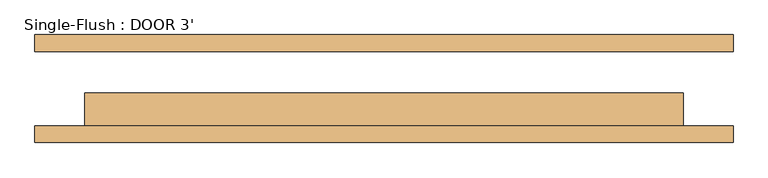
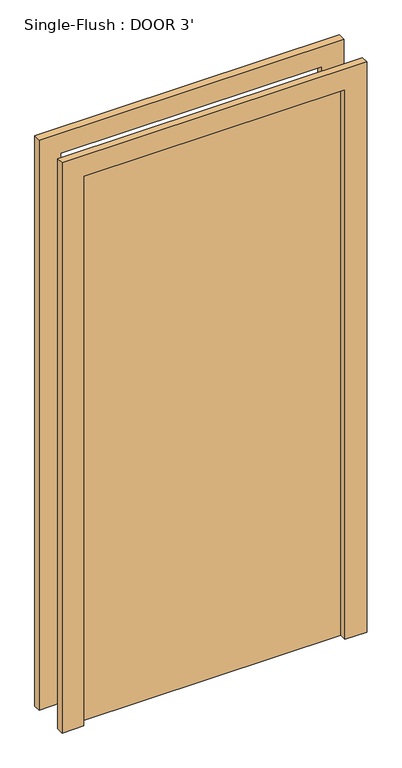
"""IFC4 building model written with IfcOpenShell, lengths in millimetres: door geometry, Single-Flush : DOOR 3'."""

from ifc_helpers import new_model, si_unit, frame, origin, origin_with_axes, place, context, project, spatial, polyline, outline, extrude, source, transform, mapped, element, save


def single_flush_door_3_5e62189b(model_context):
    return source(origin(), model_context, "Body", "SweptSolid", [
        extrude(outline(polyline([(2108.2, -533.4), (0.0, -533.4), (0.0, -457.2), (2032.0, -457.2), (2032.0, 457.2), (0.0, 457.2), (0.0, 533.4), (2108.2, 533.4), (2108.2, -533.4)])), frame((0.0, -82.55, 0.0), z_axis=(0.0, 1.0, 0.0), x_axis=(0.0, 0.0, 1.0)), (0.0, 0.0, 1.0), 25.4),
        extrude(outline(polyline([(2108.2, 533.4), (2108.2, -533.4), (0.0, -533.4), (0.0, -457.2), (2032.0, -457.2), (2032.0, 457.2), (0.0, 457.2), (0.0, 533.4), (2108.2, 533.4)])), frame((0.0, 57.15, 0.0), z_axis=(0.0, 1.0, 0.0), x_axis=(0.0, 0.0, 1.0)), (0.0, 0.0, 1.0), 25.4),
        extrude(outline(polyline([(457.2, -6.35), (457.2, -57.15), (-457.2, -57.15), (-457.2, -6.35), (457.2, -6.35)])), origin_with_axes(), (0.0, 0.0, 1.0), 2032.0),
    ])


if __name__ == "__main__":
    model = new_model("IFC4")
    model_context = context("Model", 3, world=origin())
    ifc_project = project(units=[si_unit("LENGTHUNIT", "METRE", prefix="MILLI")], contexts=[model_context])
    site = spatial("IfcSite", under=ifc_project)
    building = spatial("IfcBuilding", under=site)
    placement = place(None, origin())
    single_flush_door_3_shape = single_flush_door_3_5e62189b(model_context)
    element("IfcDoor", 1, ObjectType="Single-Flush : DOOR 3'", at=placement, inside=building, context=model_context, shape_type="MappedRepresentation", body=[
        mapped(single_flush_door_3_shape, transform((0.0, 0.0, 0.0), x_axis=(1.0, 0.0, 0.0), y_axis=(0.0, 1.0, 0.0), z_axis=(0.0, 0.0, 1.0))),
    ])
    save(model, "model.ifc")

# Revit data of these elements
# Type "Single-Flush : DOOR 3'"
#   Type Mark = "8"
#   Construction Type Id = "MDOOR"
#   Assembly Code = "C1020"
#   Analytic Construction = "Metal"
#   Thickness = 0' - 2"
#   Heat Transfer Coefficient (U) = 0.651978 BTU/(h·ft²·°F)
#   Height = 6' - 8"
#   Trim Projection Ext = 0' - 1"
#   Trim Projection Int = 0' - 1"
#   Trim Width = 0' - 3"
#   Width = 3' - 0"
#   Define Thermal Properties by = 1
#   Door Material = Door - Panel
#   Frame Material = Door - Frame
#   Visual Light Transmittance = 0
#   Solar Heat Gain Coefficient = 0
#   Function = (empty or 0)
#   Wall Closure = (empty or 0)
# Element 1 (IfcDoor, "Single-Flush : DOOR 3'")
#   Materials on its faces: "Door - Frame", "Door - Panel"
# Materials
#   "Door - Panel": class "Wood", colour RGB 210 159 95, transparency 0, Cost = 0
#   "Door - Frame": colour RGB 118 70 51, transparency 0, Cost = 0
